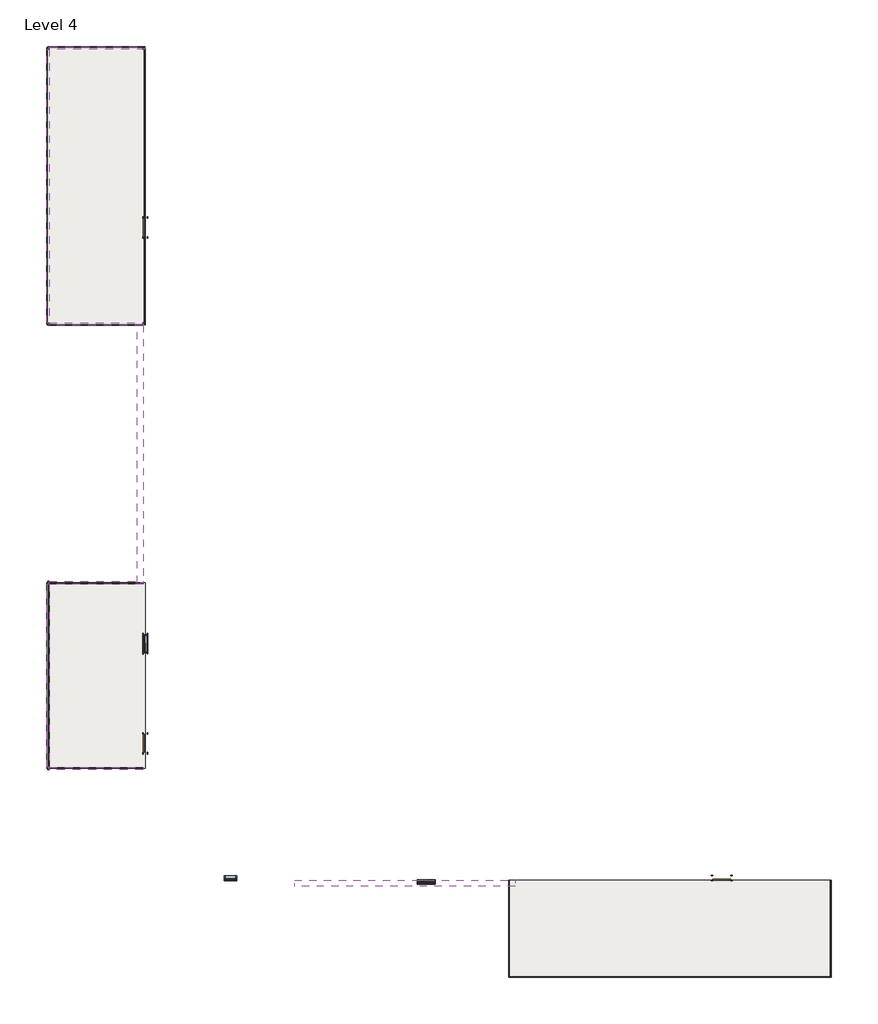
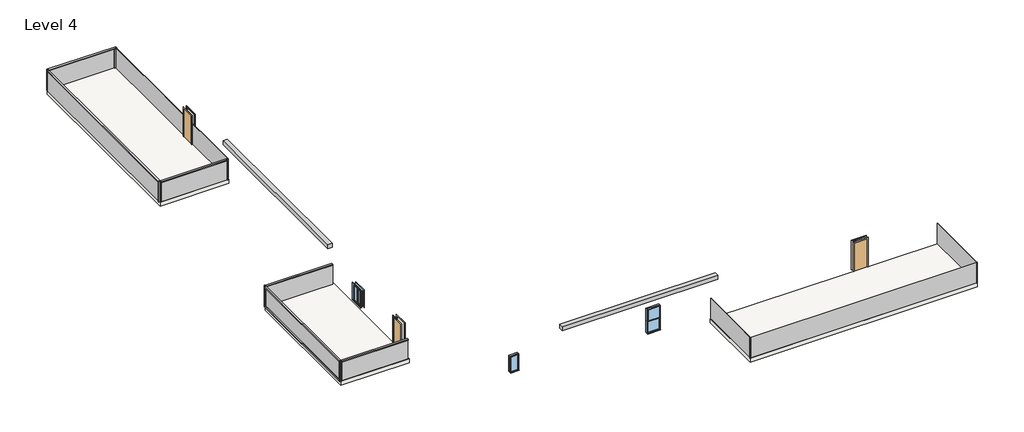
# One storey: 17 members, 10 plates, 3 doors, 3 slabs, 3 windows, 2 proxies.
"""IFC4 building model written with IfcOpenShell, lengths in millimetres."""

from ifc_helpers import new_model, si_unit, frame, origin, place, context, project, spatial, polyline, outline, extrude, transform, mapped, element, save
from components import generic_models_10_generic_models_10_788d613d, generic_models_21_generic_models_21_4b7ad0a9, door_54dd4da4, door_719f80de, member_a0ba9e48, member_4491d118, member_c8d661c8, member_35409717, member_8787ee90, member_e4af79e9, system_panel_glazed_6303489a, system_panel_glazed_dbf8c7ac, system_panel_glazed_82bc3a22, system_panel_glazed_e5b44d49, system_panel_glazed_dcdbdfd1, system_panel_glazed_281b5f8b, system_panel_glazed_ae5726c8, system_panel_glazed_7dd8e57f, window_f274a882, window_78885257, window_54100e87

model = new_model("IFC4")

# Units and contexts
model_context = context("Model", 3, world=origin())
ifc_project = project(units=[si_unit("LENGTHUNIT", "METRE", prefix="MILLI")], contexts=[model_context])

# Site, building, storey
site = spatial("IfcSite", under=ifc_project)
building = spatial("IfcBuilding", under=site)
storey = spatial("IfcBuildingStorey", under=building, Name="Level 4", Elevation=6400.8)

# Proxies
placement = place(None, origin())
generic_models_10_generic_models_10_shape = generic_models_10_generic_models_10_788d613d(model_context)
element("IfcBuildingElementProxy", 1, Name="Generic Models 10 : Generic Models 10", ObjectType="Generic Models 10 : Generic Models 10", at=placement, inside=storey, context=model_context, shape_type="MappedRepresentation", body=[
    mapped(generic_models_10_generic_models_10_shape, transform((0.0, 0.0, 0.0), x_axis=(1.0, 0.0, 0.0), y_axis=(0.0, 1.0, 0.0), z_axis=(0.0, 0.0, 1.0))),
])
generic_models_21_generic_models_21_shape = generic_models_21_generic_models_21_4b7ad0a9(model_context)
element("IfcBuildingElementProxy", 2, Name="Generic Models 21 : Generic Models 21", ObjectType="Generic Models 21 : Generic Models 21", at=placement, inside=storey, context=model_context, shape_type="MappedRepresentation", body=[
    mapped(generic_models_21_generic_models_21_shape, transform((0.0, 0.0, 0.0), x_axis=(1.0, 0.0, 0.0), y_axis=(0.0, 1.0, 0.0), z_axis=(0.0, 0.0, 1.0))),
])

# Doors
door_shape = door_54dd4da4(model_context)
element("IfcDoor", 3, ObjectType="Single-Flush : 36\" x 84\"", at=placement, inside=storey, context=model_context, shape_type="MappedRepresentation", body=[
    mapped(door_shape, transform((-15175.038074, 11818.6014639, 6400.8), x_axis=(0.0, 1.0, 0.0), y_axis=(-1.0, 0.0, 0.0), z_axis=(0.0, 0.0, 1.0))),
])
element("IfcDoor", 4, ObjectType="Single-Flush : 36\" x 84\"", at=placement, inside=storey, context=model_context, shape_type="MappedRepresentation", body=[
    mapped(door_shape, transform((-15175.038074, -14004.9915889, 6400.8), x_axis=(0.0, 1.0, 0.0), y_axis=(-1.0, 0.0, 0.0), z_axis=(0.0, 0.0, 1.0))),
])
door_2_shape = door_719f80de(model_context)
element("IfcDoor", 5, ObjectType="Single-Flush : 36\" x 84\"", at=placement, inside=storey, context=model_context, shape_type="MappedRepresentation", body=[
    mapped(door_2_shape, transform((13679.361926, -20744.1985361, 6400.8), x_axis=(1.0, 0.0, 0.0), y_axis=(0.0, 1.0, 0.0), z_axis=(0.0, 0.0, 1.0))),
])

# Members
member_shape = member_a0ba9e48(model_context)
element("IfcMember", 6, ObjectType="Rectangular Mullion : 2.5\" x 5\" rectangular", at=placement, inside=storey, context=model_context, shape_type="MappedRepresentation", body=[
    mapped(member_shape, transform((-15175.038074, 20810.2014639, 7924.8), x_axis=(0.0, 0.0, 1.0), y_axis=(0.0, -1.0, 0.0), z_axis=(1.0, 0.0, 0.0))),
])
member_2_shape = member_4491d118(model_context)
element("IfcMember", 7, ObjectType="Rectangular Mullion : 2.5\" x 5\" rectangular", at=placement, inside=storey, context=model_context, shape_type="MappedRepresentation", body=[
    mapped(member_2_shape, transform((-20051.838074, 20810.2014639, 6400.8), x_axis=(0.0, 1.0, 0.0), y_axis=(1.0, 0.0, 0.0), z_axis=(0.0, 0.0, -1.0))),
])
element("IfcMember", 8, ObjectType="Rectangular Mullion : 2.5\" x 5\" rectangular", at=placement, inside=storey, context=model_context, shape_type="MappedRepresentation", body=[
    mapped(member_2_shape, transform((-20051.838074, 6977.5785374, 6400.8), x_axis=(-1.0, 0.0, 0.0), y_axis=(0.0, 1.0, 0.0), z_axis=(0.0, 0.0, -1.0))),
])
element("IfcMember", 9, ObjectType="Rectangular Mullion : 2.5\" x 5\" rectangular", at=placement, inside=storey, context=model_context, shape_type="MappedRepresentation", body=[
    mapped(member_2_shape, transform((-20051.838074, -5966.8213044, 6400.8), x_axis=(-1.0, 0.0, 0.0), y_axis=(0.0, 1.0, 0.0), z_axis=(0.0, 0.0, -1.0))),
])
element("IfcMember", 10, ObjectType="Rectangular Mullion : 2.5\" x 5\" rectangular", at=placement, inside=storey, context=model_context, shape_type="MappedRepresentation", body=[
    mapped(member_2_shape, transform((-20051.838074, 20810.2014639, 7924.8), x_axis=(-1.0, 0.0, 0.0), y_axis=(0.0, -1.0, 0.0), z_axis=(0.0, 0.0, 1.0))),
])
element("IfcMember", 11, ObjectType="Rectangular Mullion : 2.5\" x 5\" rectangular", at=placement, inside=storey, context=model_context, shape_type="MappedRepresentation", body=[
    mapped(member_2_shape, transform((-20051.838074, 6977.5785374, 7924.8), x_axis=(0.0, -1.0, 0.0), y_axis=(1.0, 0.0, 0.0), z_axis=(0.0, 0.0, 1.0))),
])
element("IfcMember", 12, ObjectType="Rectangular Mullion : 2.5\" x 5\" rectangular", at=placement, inside=storey, context=model_context, shape_type="MappedRepresentation", body=[
    mapped(member_2_shape, transform((-15238.538074, 6977.5785374, 7924.8), x_axis=(1.0, 0.0, 0.0), y_axis=(0.0, 1.0, 0.0), z_axis=(0.0, 0.0, 1.0))),
])
element("IfcMember", 13, ObjectType="Rectangular Mullion : 2.5\" x 5\" rectangular", at=placement, inside=storey, context=model_context, shape_type="MappedRepresentation", body=[
    mapped(member_2_shape, transform((-20051.838074, -15263.2213044, 7924.8), x_axis=(-1.0, 0.0, 0.0), y_axis=(0.0, -1.0, 0.0), z_axis=(0.0, 0.0, 1.0))),
])
element("IfcMember", 14, ObjectType="Rectangular Mullion : 2.5\" x 5\" rectangular", at=placement, inside=storey, context=model_context, shape_type="MappedRepresentation", body=[
    mapped(member_2_shape, transform((-15238.538074, 20810.2014639, 7924.8), x_axis=(0.0, 1.0, 0.0), y_axis=(-1.0, 0.0, 0.0), z_axis=(0.0, 0.0, 1.0))),
])
member_3_shape = member_c8d661c8(model_context)
element("IfcMember", 15, ObjectType="Rectangular Mullion : 2.5\" x 5\" rectangular", at=placement, inside=storey, context=model_context, shape_type="MappedRepresentation", body=[
    mapped(member_3_shape, transform((-20051.838074, 20746.7014639, 7924.8), x_axis=(0.0, 0.0, 1.0), y_axis=(1.0, 0.0, 0.0), z_axis=(0.0, 1.0, 0.0))),
])
member_4_shape = member_35409717(model_context)
element("IfcMember", 16, ObjectType="Rectangular Mullion : 2.5\" x 5\" rectangular", at=placement, inside=storey, context=model_context, shape_type="MappedRepresentation", body=[
    mapped(member_4_shape, transform((-19988.338074, 6977.5785374, 7924.8), x_axis=(0.0, 0.0, 1.0), y_axis=(0.0, 1.0, 0.0), z_axis=(-1.0, 0.0, 0.0))),
])
member_5_shape = member_8787ee90(model_context)
element("IfcMember", 17, ObjectType="Rectangular Mullion : 2.5\" x 5\" rectangular", at=placement, inside=storey, context=model_context, shape_type="MappedRepresentation", body=[
    mapped(member_5_shape, transform((-20051.838074, -15199.7213044, 7924.8), x_axis=(0.0, 0.0, 1.0), y_axis=(-1.0, 0.0, 0.0), z_axis=(0.0, -1.0, 0.0))),
])
element("IfcMember", 18, ObjectType="Rectangular Mullion : 2.5\" x 5\" rectangular", at=placement, inside=storey, context=model_context, shape_type="MappedRepresentation", body=[
    mapped(member_5_shape, transform((-20051.838074, -6030.3213044, 6400.8), x_axis=(0.0, 0.0, -1.0), y_axis=(-1.0, 0.0, 0.0), z_axis=(0.0, 1.0, 0.0))),
])
element("IfcMember", 19, ObjectType="Rectangular Mullion : 2.5\" x 5\" rectangular", at=placement, inside=storey, context=model_context, shape_type="MappedRepresentation", body=[
    mapped(member_2_shape, transform((-20051.838074, -15263.2213044, 6400.8), x_axis=(0.0, -1.0, 0.0), y_axis=(-1.0, 0.0, 0.0), z_axis=(0.0, 0.0, -1.0))),
])
element("IfcMember", 20, ObjectType="Rectangular Mullion : 2.5\" x 5\" rectangular", at=placement, inside=storey, context=model_context, shape_type="MappedRepresentation", body=[
    mapped(member_2_shape, transform((-20051.838074, -5966.8213044, 7924.8), x_axis=(0.0, 1.0, 0.0), y_axis=(-1.0, 0.0, 0.0), z_axis=(0.0, 0.0, 1.0))),
])
member_6_shape = member_e4af79e9(model_context)
element("IfcMember", 21, ObjectType="Rectangular Mullion : 2.5\" x 5\" rectangular", at=placement, inside=storey, context=model_context, shape_type="MappedRepresentation", body=[
    mapped(member_6_shape, transform((-19988.338074, -5966.8213044, 7924.8), x_axis=(0.0, 0.0, 1.0), y_axis=(0.0, 1.0, 0.0), z_axis=(-1.0, 0.0, 0.0))),
])
element("IfcMember", 22, ObjectType="Rectangular Mullion : 2.5\" x 5\" rectangular", at=placement, inside=storey, context=model_context, shape_type="MappedRepresentation", body=[
    mapped(member_6_shape, transform((-15276.638074, -15263.2213044, 7924.8), x_axis=(0.0, 0.0, 1.0), y_axis=(0.0, -1.0, 0.0), z_axis=(1.0, 0.0, 0.0))),
])

# Plates
system_panel_glazed_shape = system_panel_glazed_6303489a(model_context)
element("IfcPlate", 23, ObjectType="System Panel : Glazed", at=placement, inside=storey, context=model_context, shape_type="MappedRepresentation", body=[
    mapped(system_panel_glazed_shape, transform((3011.361926, -23284.1985361, 6400.8), x_axis=(0.0, -1.0, 0.0), y_axis=(1.0, 0.0, 0.0), z_axis=(0.0, 0.0, 1.0))),
])
element("IfcPlate", 24, ObjectType="System Panel : Glazed", at=placement, inside=storey, context=model_context, shape_type="MappedRepresentation", body=[
    mapped(system_panel_glazed_shape, transform((19165.761926, -23284.1985361, 6400.8), x_axis=(0.0, 1.0, 0.0), y_axis=(-1.0, 0.0, 0.0), z_axis=(0.0, 0.0, 1.0))),
])
system_panel_glazed_2_shape = system_panel_glazed_dbf8c7ac(model_context)
element("IfcPlate", 25, ObjectType="System Panel : Glazed", at=placement, inside=storey, context=model_context, shape_type="MappedRepresentation", body=[
    mapped(system_panel_glazed_2_shape, transform((11088.561926, -25722.5985361, 6400.8), x_axis=(1.0, 0.0, 0.0), y_axis=(0.0, 1.0, 0.0), z_axis=(0.0, 0.0, 1.0))),
])
system_panel_glazed_3_shape = system_panel_glazed_82bc3a22(model_context)
element("IfcPlate", 26, ObjectType="System Panel : Glazed", at=placement, inside=storey, context=model_context, shape_type="MappedRepresentation", body=[
    mapped(system_panel_glazed_3_shape, transform((-17581.688074, 20810.2014639, 6400.8), x_axis=(1.0, 0.0, 0.0), y_axis=(0.0, 1.0, 0.0), z_axis=(0.0, 0.0, 1.0))),
])
system_panel_glazed_4_shape = system_panel_glazed_e5b44d49(model_context)
element("IfcPlate", 27, ObjectType="System Panel : Glazed", at=placement, inside=storey, context=model_context, shape_type="MappedRepresentation", body=[
    mapped(system_panel_glazed_4_shape, transform((-20051.838074, 13893.8900007, 6400.8), x_axis=(0.0, 1.0, 0.0), y_axis=(-1.0, 0.0, 0.0), z_axis=(0.0, 0.0, 1.0))),
])
system_panel_glazed_5_shape = system_panel_glazed_dcdbdfd1(model_context)
element("IfcPlate", 28, ObjectType="System Panel : Glazed", at=placement, inside=storey, context=model_context, shape_type="MappedRepresentation", body=[
    mapped(system_panel_glazed_5_shape, transform((-17645.188074, 6977.5785374, 6400.8), x_axis=(-1.0, 0.0, 0.0), y_axis=(0.0, -1.0, 0.0), z_axis=(0.0, 0.0, 1.0))),
])
system_panel_glazed_6_shape = system_panel_glazed_281b5f8b(model_context)
element("IfcPlate", 29, ObjectType="System Panel : Glazed", at=placement, inside=storey, context=model_context, shape_type="MappedRepresentation", body=[
    mapped(system_panel_glazed_6_shape, transform((-15238.538074, 13862.1400007, 6400.8), x_axis=(0.0, -1.0, 0.0), y_axis=(1.0, 0.0, 0.0), z_axis=(0.0, 0.0, 1.0))),
])
system_panel_glazed_7_shape = system_panel_glazed_ae5726c8(model_context)
element("IfcPlate", 30, ObjectType="System Panel : Glazed", at=placement, inside=storey, context=model_context, shape_type="MappedRepresentation", body=[
    mapped(system_panel_glazed_7_shape, transform((-20051.838074, -10615.0213044, 6464.3), x_axis=(0.0, -1.0, 0.0), y_axis=(1.0, 0.0, 0.0), z_axis=(0.0, 0.0, 1.0))),
])
system_panel_glazed_8_shape = system_panel_glazed_7dd8e57f(model_context)
element("IfcPlate", 31, ObjectType="System Panel : Glazed", at=placement, inside=storey, context=model_context, shape_type="MappedRepresentation", body=[
    mapped(system_panel_glazed_8_shape, transform((-17632.488074, -5966.8213044, 6400.8), x_axis=(-1.0, 0.0, 0.0), y_axis=(0.0, -1.0, 0.0), z_axis=(0.0, 0.0, 1.0))),
])
element("IfcPlate", 32, ObjectType="System Panel : Glazed", at=placement, inside=storey, context=model_context, shape_type="MappedRepresentation", body=[
    mapped(system_panel_glazed_8_shape, transform((-17632.488074, -15263.2213044, 6400.8), x_axis=(1.0, 0.0, 0.0), y_axis=(0.0, 1.0, 0.0), z_axis=(0.0, 0.0, 1.0))),
])

# Slabs
element("IfcSlab", 33, ObjectType="Generic - 12\"", at=placement, inside=storey, context=model_context, shape_type="SweptSolid", body=[
    extrude(outline(polyline([(3011.361926, -20845.7985361), (19165.761926, -20845.7985361), (19165.761926, -25722.5985361), (3011.361926, -25722.5985361), (3011.361926, -20845.7985361)])), frame((0.0, 0.0, 6096.0), z_axis=(0.0, 0.0, 1.0), x_axis=(1.0, 0.0, 0.0)), (0.0, 0.0, 1.0), 304.8),
])
element("IfcSlab", 34, ObjectType="Generic - 12\"", at=placement, inside=storey, context=model_context, shape_type="SweptSolid", body=[
    extrude(outline(polyline([(-20051.838074, -15263.2213044), (-20051.838074, -5966.8213044), (-15175.038074, -5966.8213044), (-15175.038074, -15263.2213044), (-20051.838074, -15263.2213044)])), frame((0.0, 0.0, 6096.0), z_axis=(0.0, 0.0, 1.0), x_axis=(1.0, 0.0, 0.0)), (0.0, 0.0, 1.0), 304.8),
])
element("IfcSlab", 35, ObjectType="Generic - 12\"", at=placement, inside=storey, context=model_context, shape_type="SweptSolid", body=[
    extrude(outline(polyline([(-20051.838074, 20810.2014639), (-15175.038074, 20810.2014639), (-15175.038074, 6941.8014639), (-20051.838074, 6941.8014639), (-20051.838074, 20810.2014639)])), frame((0.0, 0.0, 6096.0), z_axis=(0.0, 0.0, 1.0), x_axis=(1.0, 0.0, 0.0)), (0.0, 0.0, 1.0), 304.8),
])

# Windows
window_shape = window_f274a882(model_context)
element("IfcWindow", 36, ObjectType="Double Hung : 36\" x 72\"", at=placement, inside=storey, context=model_context, shape_type="MappedRepresentation", body=[
    mapped(window_shape, transform((-1103.438074, -20921.9985361, 6665.1958658), x_axis=(-1.0, 0.0, 0.0), y_axis=(0.0, -1.0, 0.0), z_axis=(0.0, 0.0, 1.0))),
])
window_2_shape = window_78885257(model_context)
element("IfcWindow", 37, ObjectType="Instance - Fixed : 24\" x 48\"", at=placement, inside=storey, context=model_context, shape_type="MappedRepresentation", body=[
    mapped(window_2_shape, transform((-10945.938074, -20744.1985361, 6400.8), x_axis=(-1.0, 0.0, 0.0), y_axis=(0.0, -1.0, 0.0), z_axis=(0.0, 0.0, 1.0))),
])
window_3_shape = window_54100e87(model_context)
element("IfcWindow", 38, ObjectType="Slider with Trim : 36\" x 48\"", at=placement, inside=storey, context=model_context, shape_type="MappedRepresentation", body=[
    mapped(window_3_shape, transform((-15175.038074, -9014.8213044, 5852.772861), x_axis=(0.0, 1.0, 0.0), y_axis=(-1.0, 0.0, 0.0), z_axis=(0.0, 0.0, 1.0))),
])

save(model, "model.ifc")

# Revit data of these elements
# Type "Single-Flush : 36\" x 84\""
#   Type Mark = "1"
#   Construction Type Id = "MDOOR"
#   Assembly Code = "C1020"
#   Analytic Construction = "Metal"
#   Thickness = 0' - 2"
#   Heat Transfer Coefficient (U) = 0.651978 BTU/(h·ft²·°F)
#   Height = 7' - 0"
#   Trim Projection Ext = 0' - 1"
#   Trim Projection Int = 0' - 1"
#   Trim Width = 0' - 3"
#   Width = 3' - 0"
#   Define Thermal Properties by = 1
#   Door Material = Door - Panel
#   Frame Material = Door - Frame
#   Visual Light Transmittance = 0
#   Solar Heat Gain Coefficient = 0
#   Function = (empty or 0)
#   Wall Closure = (empty or 0)
# Type "Rectangular Mullion : 2.5\" x 5\" rectangular"
#   built-in parameter 1007304 = 0.416667 (stored number, unit not read)
#   built-in parameter 1007301 = 0.104167 (stored number, unit not read)
#   built-in parameter 1007300 = 0.104167 (stored number, unit not read)
# Type "System Panel : Glazed"
#   Construction Type Id = "GSP4R"
#   Analytic Construction = "1/8 in Pilkington single glazing"
#   Visual Light Transmittance = 0.9
#   Solar Heat Gain Coefficient = 0.86
#   Heat Transfer Coefficient (U) = 1.18115 BTU/(h·ft²·°F)
# Type "Generic - 12\""
#   Assembly Code = "B1010"
#   Function = 0
#   Layers, outside or top first: 1' - 0" no material (function 1)
# Type "Double Hung : 36\" x 72\""
#   Type Mark = "18"
#   Construction Type Id = "GSP4R"
#   Assembly Code = "B2020100"
#   Analytic Construction = "1/8 in Pilkington single glazing"
#   Visual Light Transmittance = 0.9
#   Solar Heat Gain Coefficient = 0.78
#   Heat Transfer Coefficient (U) = 0.6496 BTU/(h·ft²·°F)
#   Height = 6' - 0"
#   Default Sill Height = 1' - 0"
#   Width = 3' - 0"
#   Window Inset = 0' - 0 3/4"
#   Define Thermal Properties by = 1
#   Glass Pane Material = Glass
#   Sash Material = Sash
#   Description = (empty or 0)
#   Wall Closure = (empty or 0)
# Type "Instance - Fixed : 24\" x 48\""
#   Type Mark = "19"
#   Construction Type Id = "GSP4R"
#   Assembly Code = "B2020100"
#   Analytic Construction = "1/8 in Pilkington single glazing"
#   Visual Light Transmittance = 0.9
#   Thermal Resistance (R) = 0.8466 (h·ft²·°F)/BTU
#   Solar Heat Gain Coefficient = 0.86
#   Heat Transfer Coefficient (U) = 1.1812 BTU/(h·ft²·°F)
#   Height [instance default] = 4' - 0"
#   Default Sill Height = 3' - 0"
#   Width [instance default] = 2' - 0"
#   Window Inset = 0' - 0 3/4"
#   Define Thermal Properties by = 1
#   Glass Pane Material = Glass
#   Sash Material = Sash
#   Wall Closure = (empty or 0)
# Type "Slider with Trim : 36\" x 48\""
#   Type Mark = "22"
#   Construction Type Id = "GSP4R"
#   Assembly Code = "B2020100"
#   Analytic Construction = "1/8 in Pilkington single glazing"
#   Visual Light Transmittance = 0.9
#   Solar Heat Gain Coefficient = 0.78
#   Heat Transfer Coefficient (U) = 0.6496 BTU/(h·ft²·°F)
#   Height = 4' - 0"
#   Default Sill Height = 3' - 0"
#   Trim Projection - Ext. = 0' - 0 3/4"
#   Trim Projection - Int. = 0' - 0 3/4"
#   Trim Width - Exterior = 0' - 3 1/2"
#   Trim Width - Interior = 0' - 3 1/2"
#   Width = 3' - 0"
#   Window Inset = 0' - 0 3/4"
#   Define Thermal Properties by = 1
#   Glass Pane Material = Glass
#   Sash Material = Sash
#   Trim Exterior Material = Trim
#   Trim Interior Material = Trim
#   Wall Closure = (empty or 0)
# Element 1 (IfcBuildingElementProxy, "Generic Models 10 : Generic Models 10")
#   Phase Created = New Construction
# Element 2 (IfcBuildingElementProxy, "Generic Models 21 : Generic Models 21")
#   Phase Created = New Construction
# Elements 3, 4, 5 (IfcDoor, "Single-Flush : 36\" x 84\"")
#   Phase Created = New Construction
#   Materials on its faces: "Door - Frame", "Door - Panel"
# Elements 6, 7, 8, 9, 10, 11, 12, 13, 14, 15, 16, 17, 18, 19, 20, 21, 22 (IfcMember, "Rectangular Mullion : 2.5\" x 5\" rectangular")
#   Phase Created = New Construction
#   Materials on its faces: "Aluminum"
# Elements 23, 24, 25, 26, 27, 28, 29, 30, 31, 32 (IfcPlate, "System Panel : Glazed")
#   Phase Created = New Construction
#   Materials on its faces: "Glass"
# Elements 33, 34, 35 (IfcSlab, "Generic - 12\"")
#   built-in parameter 1001955 = 3.14159 (stored number, unit not read)
#   Height Offset From Level = 0' - 0"
#   Phase Created = New Construction
#   Materials on its faces: "Default Floor"
# Element 36 (IfcWindow, "Double Hung : 36\" x 72\"")
#   Mark = "10"
#   Phase Created = New Construction
#   Materials on its faces: "Sash", "Glass"
# Element 37 (IfcWindow, "Instance - Fixed : 24\" x 48\"")
#   Mark = "21"
#   Width = 2' - 0"
#   Height = 4' - 0"
#   Phase Created = New Construction
#   Materials on its faces: "Sash", "Glass"
# Element 38 (IfcWindow, "Slider with Trim : 36\" x 48\"")
#   Mark = "43"
#   Phase Created = New Construction
#   Materials on its faces: "Sash", "Trim", "Glass"
# Materials
#   "Door - Panel": class "Wood", colour RGB 210 159 95, transparency 0
#   "Door - Frame": colour RGB 118 70 51, transparency 0
#   "Glass": class "Glass", colour RGB 0 128 192, transparency 0.75, Description = "Soda Lime Glass", Cost = 0
#   "Sash": class "Wood", colour RGB 224 178 126, transparency 0
#   "Trim": class "Wood", colour RGB 224 178 126, transparency 0
#   "Aluminum": class "Metal", colour RGB 247 247 247, transparency 0, Description = "Aluminum 6061", Cost = 0
#   "Default Floor": colour RGB 128 128 128, transparency 0
